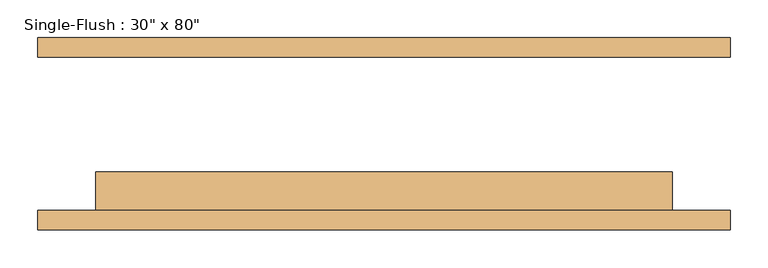
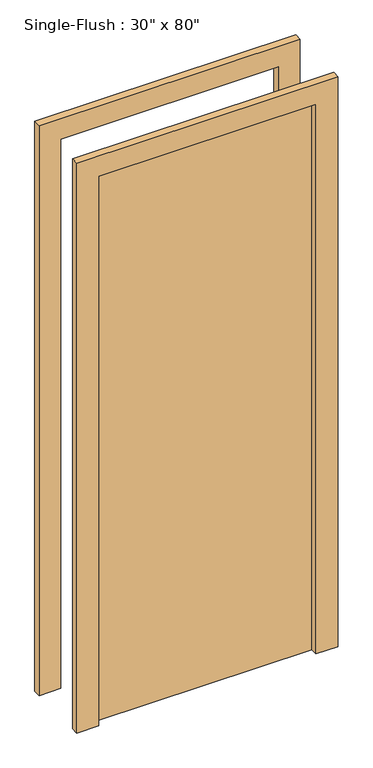
"""IFC4 building model written with IfcOpenShell, lengths in millimetres: door geometry."""

from ifc_helpers import new_model, si_unit, frame, origin, origin_with_axes, place, context, project, spatial, polyline, outline, extrude, source, transform, mapped, element, save


def door_53b1b562(model_context):
    return source(origin(), model_context, "Body", "SweptSolid", [
        extrude(outline(polyline([(2108.2, -457.2), (0.0, -457.2), (0.0, -381.0), (2032.0, -381.0), (2032.0, 381.0), (0.0, 381.0), (0.0, 457.2), (2108.2, 457.2), (2108.2, -457.2)])), frame((0.0, -127.0, 0.0), z_axis=(0.0, 1.0, 0.0), x_axis=(0.0, 0.0, 1.0)), (0.0, 0.0, 1.0), 25.4),
        extrude(outline(polyline([(2108.2, 457.2), (2108.2, -457.2), (0.0, -457.2), (0.0, -381.0), (2032.0, -381.0), (2032.0, 381.0), (0.0, 381.0), (0.0, 457.2), (2108.2, 457.2)])), frame((0.0, 101.6, 0.0), z_axis=(0.0, 1.0, 0.0), x_axis=(0.0, 0.0, 1.0)), (0.0, 0.0, 1.0), 25.4),
        extrude(outline(polyline([(381.0, -50.8), (381.0, -101.6), (-381.0, -101.6), (-381.0, -50.8), (381.0, -50.8)])), origin_with_axes(), (0.0, 0.0, 1.0), 2032.0),
    ])


if __name__ == "__main__":
    model = new_model("IFC4")
    model_context = context("Model", 3, world=origin())
    ifc_project = project(units=[si_unit("LENGTHUNIT", "METRE", prefix="MILLI")], contexts=[model_context])
    site = spatial("IfcSite", under=ifc_project)
    building = spatial("IfcBuilding", under=site)
    placement = place(None, origin())
    door_shape = door_53b1b562(model_context)
    element("IfcDoor", 1, ObjectType="Single-Flush : 30\" x 80\"", at=placement, inside=building, context=model_context, shape_type="MappedRepresentation", body=[
        mapped(door_shape, transform((0.0, 0.0, 0.0), x_axis=(1.0, 0.0, 0.0), y_axis=(0.0, 1.0, 0.0), z_axis=(0.0, 0.0, 1.0))),
    ])
    save(model, "model.ifc")

# Revit data of these elements
# Type "Single-Flush : 30\" x 80\""
#   Type Mark = "5"
#   Assembly Code = "C1020"
#   Thickness = 0' - 2"
#   Height = 6' - 8"
#   Trim Projection Ext = 0' - 1"
#   Trim Projection Int = 0' - 1"
#   Trim Width = 0' - 3"
#   Width = 2' - 6"
#   Door Material = Door - Panel
#   Frame Material = Door - Frame
#   Function = (empty or 0)
#   Wall Closure = (empty or 0)
# Element 1 (IfcDoor, "Single-Flush : 30\" x 80\"")
#   Materials on its faces: "Door - Frame", "Door - Panel"
# Materials
#   "Door - Panel": class "Wood", colour RGB 114 82 51, transparency 0
#   "Door - Frame": colour RGB 153 76 43, transparency 0
